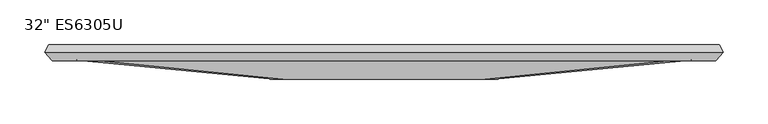
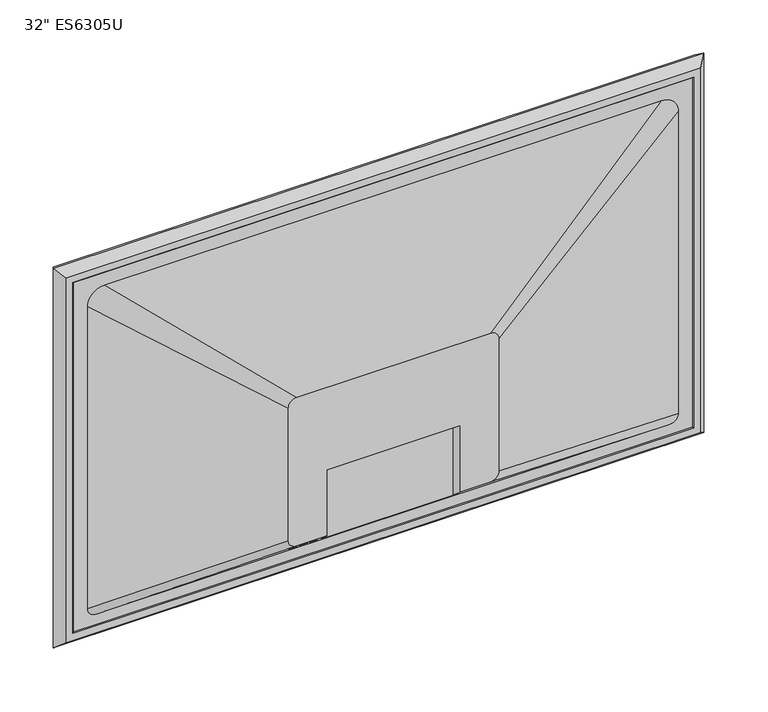
"""IFC4 building model written with IfcOpenShell, lengths in millimetres: proxy geometry."""

from ifc_helpers import new_model, si_unit, point, frame, origin, place, context, project, spatial, polyline, circle_curve, ellipse_curve, trimmed, outline, extrude, faceted_brep, source, transform, mapped, element, save
from ifc_brep_helpers import plane_surface, revolved_surface, extruded_surface, spline_surface, advanced_brep


def proxy_88c96ab6(model_context):
    return source(origin(), model_context, "Body", "SolidModel", [
        extrude(outline(polyline([(-245.0, 182.3), (495.0, 182.3), (495.0, 166.3), (-245.0, 166.3), (-245.0, 182.3)])), frame((0.0, 0.0, 1604.8), z_axis=(0.0, 0.0, 1.0), x_axis=(1.0, 0.0, 0.0)), (0.0, 0.0, 1.0), 448.0),
        advanced_brep(
        [(-205.0, 166.3, 2032.8), (455.0, 166.3, 2032.8), (475.0, 166.3, 2012.8), (475.0, 166.3, 1634.8), (465.0, 166.3, 1624.8), (-215.0, 166.3, 1624.8), (-225.0, 166.3, 1634.8), (-225.0, 166.3, 2012.8), (11.6666667, 144.3, 1828.8), (1.6666667, 144.3, 1818.8), (1.6666667, 144.3, 1654.8), (11.6666667, 144.3, 1644.8), (46.6666667, 144.3, 1644.8), (46.6666667, 144.3, 1726.8), (203.3333333, 144.3, 1726.8), (203.3333333, 144.3, 1644.8), (238.3333333, 144.3, 1644.8), (248.3333333, 144.3, 1654.8), (248.3333333, 144.3, 1818.8), (238.3333333, 144.3, 1828.8), (203.3333333, 160.3, 1630.2545455), (46.6666667, 160.3, 1630.2545455), (20.843372, 154.3, 1635.7090909), (28.843372, 154.3, 1635.7090909), (32.8393281, 154.3, 1635.7090909), (40.8393281, 154.3, 1635.7090909), (8.7618145, 154.3, 1635.7090909), (16.7618145, 154.3, 1635.7090909), (203.3333333, 160.3, 1726.8), (46.6666667, 160.3, 1726.8), (20.843372, 154.3, 1656.8), (24.843372, 154.3, 1656.8), (28.843372, 154.3, 1656.8), (32.8393281, 154.3, 1656.8), (36.8393281, 154.3, 1656.8), (40.8393281, 154.3, 1656.8), (8.7618145, 154.3, 1656.8), (12.7618145, 154.3, 1656.8), (16.7618145, 154.3, 1656.8)],
        [
            (0, 1),
            (1, 2, circle_curve(frame((455.0, 166.3, 2012.8), z_axis=(0.0, 1.0, 0.0), x_axis=(-1.0, 0.0, 0.0)), 20.0)),
            (2, 3),
            (3, 4, circle_curve(frame((465.0, 166.3, 1634.8), z_axis=(0.0, 1.0, 0.0), x_axis=(-1.0, 0.0, 0.0)), 10.0)),
            (4, 5),
            (5, 6, circle_curve(frame((-215.0, 166.3, 1634.8), z_axis=(0.0, 1.0, 0.0), x_axis=(-1.0, 0.0, 0.0)), 10.0)),
            (6, 7),
            (7, 0, circle_curve(frame((-205.0, 166.3, 2012.8), z_axis=(0.0, 1.0, 0.0), x_axis=(-1.0, 0.0, 0.0)), 20.0)),
            (8, 9, circle_curve(frame((11.6666667, 144.3, 1818.8), z_axis=(0.0, -1.0, 0.0), x_axis=(-1.0, 0.0, 0.0)), 10.0)),
            (9, 10),
            (10, 11, circle_curve(frame((11.6666667, 144.3, 1654.8), z_axis=(0.0, -1.0, 0.0), x_axis=(-1.0, 0.0, 0.0)), 10.0)),
            (11, 12),
            (12, 13),
            (13, 14),
            (14, 15),
            (15, 16),
            (16, 17, circle_curve(frame((238.3333333, 144.3, 1654.8), z_axis=(0.0, -1.0, 0.0), x_axis=(-1.0, 0.0, 0.0)), 10.0)),
            (17, 18),
            (18, 19, circle_curve(frame((238.3333333, 144.3, 1818.8), z_axis=(0.0, -1.0, 0.0), x_axis=(-1.0, 0.0, 0.0)), 10.0)),
            (19, 8),
            (0, 8),
            (19, 1),
            (18, 2),
            (17, 3),
            (16, 4),
            (15, 20),
            (20, 21),
            (21, 12),
            (11, 5),
            (22, 23, ellipse_curve(frame((24.843372, 154.3, 1635.7090909), z_axis=(0.0, 0.6726727939965482, 0.7399400733957293), x_axis=(0.0, 0.7399400733957292, -0.6726727939965484)), 5.4058432, 4.0)),
            (23, 22, ellipse_curve(frame((24.843372, 154.3, 1635.7090909), z_axis=(0.0, 0.6726727939965482, 0.7399400733957293), x_axis=(0.0, 0.7399400733957292, -0.6726727939965484)), 5.4058432, 4.0)),
            (24, 25, ellipse_curve(frame((36.8393281, 154.3, 1635.7090909), z_axis=(0.0, 0.6726727939965482, 0.7399400733957293), x_axis=(0.0, 0.7399400733957292, -0.6726727939965484)), 5.4058432, 4.0)),
            (25, 24, ellipse_curve(frame((36.8393281, 154.3, 1635.7090909), z_axis=(0.0, 0.6726727939965482, 0.7399400733957293), x_axis=(0.0, 0.7399400733957292, -0.6726727939965484)), 5.4058432, 4.0)),
            (26, 27, ellipse_curve(frame((12.7618145, 154.3, 1635.7090909), z_axis=(0.0, 0.6726727939965482, 0.7399400733957293), x_axis=(0.0, 0.7399400733957292, -0.6726727939965484)), 5.4058432, 4.0)),
            (27, 26, ellipse_curve(frame((12.7618145, 154.3, 1635.7090909), z_axis=(0.0, 0.6726727939965482, 0.7399400733957293), x_axis=(0.0, 0.7399400733957292, -0.6726727939965484)), 5.4058432, 4.0)),
            (10, 6),
            (9, 7),
            (28, 29),
            (29, 21),
            (20, 28),
            (28, 14),
            (13, 29),
            (30, 31),
            (31, 32),
            (32, 30, circle_curve(frame((24.843372, 154.3, 1656.8), z_axis=(0.0, 0.0, -1.0), x_axis=(1.0, 0.0, 0.0)), 4.0)),
            (30, 32, circle_curve(frame((24.843372, 154.3, 1656.8), z_axis=(0.0, 0.0, -1.0), x_axis=(1.0, 0.0, 0.0)), 4.0)),
            (32, 23),
            (22, 30),
            (33, 34),
            (34, 35),
            (35, 33, circle_curve(frame((36.8393281, 154.3, 1656.8), z_axis=(0.0, 0.0, -1.0), x_axis=(1.0, 0.0, 0.0)), 4.0)),
            (33, 35, circle_curve(frame((36.8393281, 154.3, 1656.8), z_axis=(0.0, 0.0, -1.0), x_axis=(1.0, 0.0, 0.0)), 4.0)),
            (35, 25),
            (24, 33),
            (36, 37),
            (37, 38),
            (38, 36, circle_curve(frame((12.7618145, 154.3, 1656.8), z_axis=(0.0, 0.0, -1.0), x_axis=(1.0, 0.0, 0.0)), 4.0)),
            (36, 38, circle_curve(frame((12.7618145, 154.3, 1656.8), z_axis=(0.0, 0.0, -1.0), x_axis=(1.0, 0.0, 0.0)), 4.0)),
            (38, 27),
            (26, 36),
        ],
        [
            plane_surface(frame((125.0, 166.3, 1826.3), z_axis=(0.0, 1.0, 0.0), x_axis=(1.0, 0.0, 0.0))),
            plane_surface(frame((125.0, 144.3, 1736.8), z_axis=(0.0, -1.0, 0.0), x_axis=(1.0, 0.0, 0.0))),
            plane_surface(frame((125.0, 144.3, 1828.8), z_axis=(0.0, -0.9942351648103037, 0.10722143934227049), x_axis=(1.0, 0.0, 0.0))),
            spline_surface(2, 1, [[(238.3333333, 144.3, 1828.8), (455.0, 166.3, 2032.8)], [(248.3333333, 144.3, 1828.8), (475.0, 166.3, 2032.8)], [(248.3333333, 144.3, 1818.8), (475.0, 166.3, 2012.8)]], [3, 3], [2, 2], [0.0, 1.0], [0.0, 1.0], weights=[[1.0, 1.0], [0.7071067811865476, 0.7071067811865476], [1.0, 1.0]]),
            plane_surface(frame((248.3333333, 144.3, 1736.8), z_axis=(0.09660486119908186, -0.9953228123542162, 0.0), x_axis=(0.0, 0.0, -1.0))),
            extruded_surface(trimmed(circle_curve(frame((238.3333333, 144.3, 1654.8), z_axis=(0.0, 1.0, 0.0), x_axis=(-1.0, 0.0, 0.0)), 10.0), [point((248.3333333, 144.3, 1654.8))], [point((238.3333333, 144.3, 1644.8))], True, "CARTESIAN"), (226.6666667, 22.0, -20.0), 228.60835022564004),
            plane_surface(frame((125.0, 144.3, 1644.8), z_axis=(0.0, -0.6726727939965482, -0.7399400733957293), x_axis=(-1.0, 0.0, 0.0))),
            extruded_surface(trimmed(circle_curve(frame((11.6666667, 144.3, 1654.8), z_axis=(0.0, 1.0, 0.0), x_axis=(-1.0, 0.0, 0.0)), 10.0), [point((11.6666667, 144.3, 1644.8))], [point((1.6666667, 144.3, 1654.8))], True, "CARTESIAN"), (-226.6666667, 22.0, -20.0), 228.60835022564004),
            plane_surface(frame((1.6666667, 144.3, 1736.8), z_axis=(-0.09660486119908743, -0.9953228123542156, 0.0), x_axis=(0.0, 0.0, 1.0))),
            spline_surface(2, 1, [[(1.6666667, 144.3, 1818.8), (-225.0, 166.3, 2012.8)], [(1.6666667000000004, 144.3, 1828.8), (-225.0, 166.3, 2032.8)], [(11.6666667, 144.3, 1828.8), (-205.0, 166.3, 2032.8)]], [3, 3], [2, 2], [0.0, 1.0], [0.0, 1.0], weights=[[1.0, 1.0], [0.7071067811865476, 0.7071067811865476], [1.0, 1.0]]),
            plane_surface(frame((203.3333333, 160.3, 1726.8), z_axis=(0.0, -1.0, 0.0), x_axis=(1.0, 0.0, 0.0))),
            plane_surface(frame((46.6666667, 160.3, 1726.8), z_axis=(0.0, 0.0, -1.0), x_axis=(0.0, -1.0, 0.0))),
            plane_surface(frame((203.3333333, 160.3, 1726.8), z_axis=(-1.0, 0.0, 0.0), x_axis=(0.0, -1.0, 0.0))),
            plane_surface(frame((46.6666667, 160.3, 1604.8), z_axis=(1.0, 0.0, 0.0), x_axis=(0.0, -1.0, 0.0))),
            plane_surface(frame((24.843372, 154.3, 1656.8), z_axis=(0.0, 0.0, -1.0), x_axis=(1.0, 0.0, 0.0))),
            revolved_surface(polyline([(28.843372, 154.3, 1632.0727272507488), (28.843372, 154.3, 1656.8)]), (24.843372, 154.3, 1550.9439481), (0.0, 0.0, -1.0)),
            plane_surface(frame((36.8393281, 154.3, 1656.8), z_axis=(0.0, 0.0, -1.0), x_axis=(1.0, 0.0, 0.0))),
            revolved_surface(polyline([(40.8393281, 154.3, 1632.0727272507488), (40.8393281, 154.3, 1656.8)]), (36.8393281, 154.3, 1550.9439481), (0.0, 0.0, -1.0)),
            plane_surface(frame((12.7618145, 154.3, 1656.8), z_axis=(0.0, 0.0, -1.0), x_axis=(1.0, 0.0, 0.0))),
            revolved_surface(polyline([(16.7618145, 154.3, 1632.0727272507488), (16.7618145, 154.3, 1656.8)]), (12.7618145, 154.3, 1550.9439481), (0.0, 0.0, -1.0)),
        ],
        [
            (0, [[1, 2, 3, 4, 5, 6, 7, 8]]),
            (1, [[9, 10, 11, 12, 13, 14, 15, 16, 17, 18, 19, 20]]),
            (2, [[-1, 21, -20, 22]]),
            (3, [[-2, -22, -19, 23]]),
            (4, [[-3, -23, -18, 24]]),
            (5, [[-4, -24, -17, 25]]),
            (6, [[-5, -25, -16, 26, 27, 28, -12, 29], [30, 31], [32, 33], [34, 35]]),
            (7, [[-6, -29, -11, 36]]),
            (8, [[-7, -36, -10, 37]]),
            (9, [[-8, -37, -9, -21]]),
            (10, [[38, 39, -27, 40]]),
            (11, [[-38, 41, -14, 42]]),
            (12, [[-41, -40, -26, -15]]),
            (13, [[-42, -13, -28, -39]]),
            (14, [[43, 44, 45]]),
            (14, [[-43, 46, -44]]),
            (15, [[-45, 47, -30, 48]]),
            (15, [[-46, -48, -31, -47]]),
            (16, [[49, 50, 51]]),
            (16, [[-49, 52, -50]]),
            (17, [[-51, 53, -32, 54]]),
            (17, [[-52, -54, -33, -53]]),
            (18, [[55, 56, 57]]),
            (18, [[-55, 58, -56]]),
            (19, [[-57, 59, -34, 60]]),
            (19, [[-58, -60, -35, -59]]),
        ],
    ),
        faceted_brep([(-245.0, 182.3, 2052.8), (-245.0, 166.3, 2052.8), (-245.0, 166.3, 1604.8), (-245.0, 182.3, 1604.8), (-241.9959269, 183.3, 2049.7959269), (-240.6768394, 182.3, 2048.4768394), (-240.6768394, 182.3, 1609.1231606), (-241.9959269, 183.3, 1607.8040731), (-255.9259805, 174.7959377, 2063.7259805), (-251.0289147, 183.3, 2058.8289147), (-251.0289147, 183.3, 1598.7710853), (-255.9259805, 174.7959377, 1593.8740195), (-247.0701472, 165.3, 2054.8701472), (-247.0701472, 165.3, 1602.7298528), (-236.8560519, 166.3, 2044.6560519), (-238.5579741, 165.3, 2046.3579741), (-238.5579741, 165.3, 1611.2420259), (-236.8560519, 166.3, 1612.9439481), (495.0, 166.3, 1604.8), (495.0, 182.3, 1604.8), (490.6768394, 182.3, 1609.1231606), (491.9959269, 183.3, 1607.8040731), (501.0289147, 183.3, 1598.7710853), (505.9259805, 174.7959377, 1593.8740195), (497.0701472, 165.3, 1602.7298528), (488.5579741, 165.3, 1611.2420259), (486.8560519, 166.3, 1612.9439481), (495.0, 166.3, 2052.8), (495.0, 182.3, 2052.8), (490.6768394, 182.3, 2048.4768394), (491.9959269, 183.3, 2049.7959269), (501.0289147, 183.3, 2058.8289147), (505.9259805, 174.7959377, 2063.7259805), (497.0701472, 165.3, 2054.8701472), (488.5579741, 165.3, 2046.3579741), (486.8560519, 166.3, 2044.6560519)], [[[0, 1, 2, 3]], [[4, 5, 6, 7]], [[8, 9, 10, 11]], [[12, 8, 11, 13]], [[14, 15, 16, 17]], [[3, 2, 18, 19]], [[7, 6, 20, 21]], [[11, 10, 22, 23]], [[13, 11, 23, 24]], [[17, 16, 25, 26]], [[19, 18, 27, 28]], [[21, 20, 29, 30]], [[23, 22, 31, 32]], [[24, 23, 32, 33]], [[26, 25, 34, 35]], [[28, 27, 1, 0]], [[3, 19, 28, 0], [5, 29, 20, 6]], [[30, 29, 5, 4]], [[9, 31, 22, 10], [7, 21, 30, 4]], [[32, 31, 9, 8]], [[33, 32, 8, 12]], [[13, 24, 33, 12], [15, 34, 25, 16]], [[35, 34, 15, 14]], [[1, 27, 18, 2], [17, 26, 35, 14]]]),
    ])


if __name__ == "__main__":
    model = new_model("IFC4")
    model_context = context("Model", 3, world=origin())
    ifc_project = project(units=[si_unit("LENGTHUNIT", "METRE", prefix="MILLI")], contexts=[model_context])
    site = spatial("IfcSite", under=ifc_project)
    building = spatial("IfcBuilding", under=site)
    placement = place(None, origin())
    proxy_shape = proxy_88c96ab6(model_context)
    element("IfcBuildingElementProxy", 1, Name="32\" ES6305U", ObjectType="32\" ES6305U", at=placement, inside=building, context=model_context, shape_type="MappedRepresentation", body=[
        mapped(proxy_shape, transform((0.0, 0.0, 0.0), x_axis=(1.0, 0.0, 0.0), y_axis=(0.0, 1.0, 0.0), z_axis=(0.0, 0.0, 1.0))),
    ])
    save(model, "model.ifc")

# Revit data of these elements
# Type "32\" ES6305U"
#   URL = "http://www.samsung.com"
#   Model = "32ES6305U"
#   Manufacturer = "Samsung"
#   Description = "3D led smart tv, 6 series"
#   Width = 2' - 5.13386"
#   Placement height [instance default] = 5' - 6.92913"
#   Outputs inset = 0' - 0.3937"
#   Output size = 0' - 0.15748"
#   Inset corners = 0' - 0.3937"
#   Inset component exit = 0' - 1.77165"
#   Inset body = 0' - 0.7874"
#   Height = 1' - 5.6378"
#   Depth screen = 0' - 0.62992"
#   Depth frame edge = 0' - 0.03937"
#   Depth distance = 0' - 1.1811"
#   Depth body = 0' - 0.86614"
#   Screen material = TV Screen material
#   Frame material = TV Frame material
#   Body material = TV Body material
#   Default Elevation = 0
# Element 1 (IfcBuildingElementProxy, "32\" ES6305U")
#   Placement height = 6' - 0"
#   Materials on its faces: "TV Body material", "TV Frame material", "TV Screen material"
# Materials
#   "TV Screen material": class "Plastic", colour RGB 5 5 5, transparency 0, Description = "Plastic, generic, opaque black", Cost = 0
#   "TV Frame material": class "Metal", colour RGB 244 244 244, transparency 0, Cost = 0
#   "TV Body material": class "Plastic", colour RGB 31 31 31, transparency 0, Description = "Plastic, generic, opaque dark grey", Cost = 0
